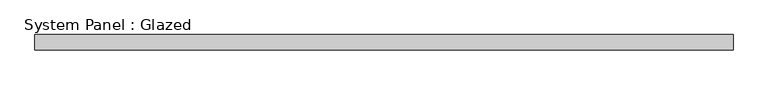
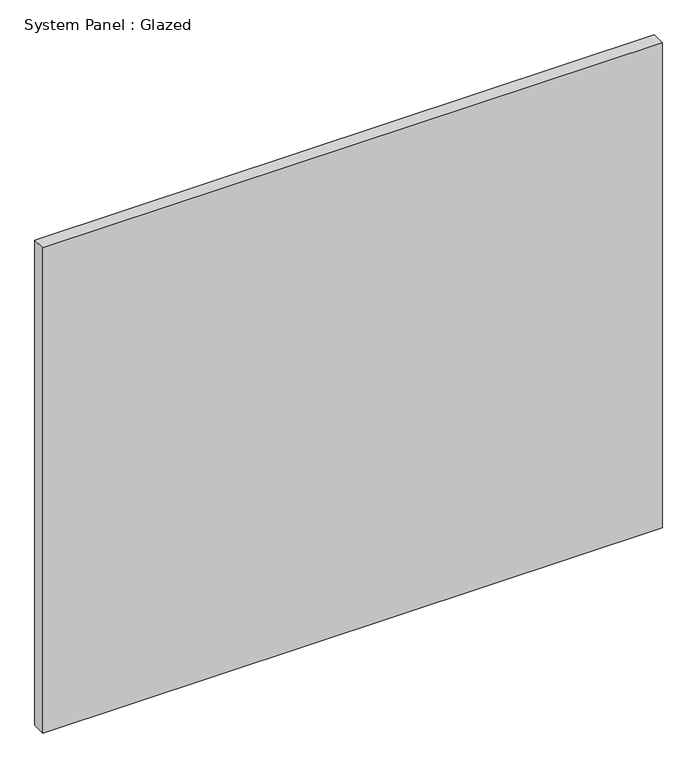
"""IFC4 building model written with IfcOpenShell, lengths in millimetres: plate geometry, System Panel : Glazed."""

from ifc_helpers import new_model, si_unit, origin, origin_with_axes, place, context, project, spatial, polyline, outline, extrude, source, transform, mapped, element, save


def system_panel_glazed_f13871fb(model_context):
    return source(origin(), model_context, "Body", "SweptSolid", [
        extrude(outline(polyline([(577.85, 19.05), (-577.85, 19.05), (-577.85, 44.45), (577.85, 44.45), (577.85, 19.05)])), origin_with_axes(), (0.0, 0.0, 1.0), 956.453622),
    ])


if __name__ == "__main__":
    model = new_model("IFC4")
    model_context = context("Model", 3, world=origin())
    ifc_project = project(units=[si_unit("LENGTHUNIT", "METRE", prefix="MILLI")], contexts=[model_context])
    site = spatial("IfcSite", under=ifc_project)
    building = spatial("IfcBuilding", under=site)
    placement = place(None, origin())
    system_panel_glazed_shape = system_panel_glazed_f13871fb(model_context)
    element("IfcPlate", 1, ObjectType="System Panel : Glazed", at=placement, inside=building, context=model_context, shape_type="MappedRepresentation", body=[
        mapped(system_panel_glazed_shape, transform((0.0, 0.0, 0.0), x_axis=(1.0, 0.0, 0.0), y_axis=(0.0, 1.0, 0.0), z_axis=(0.0, 0.0, 1.0))),
    ])
    save(model, "model.ifc")

# Revit data of these elements
# Type "System Panel : Glazed"
#   Construction Type Id = "GSP4R"
#   Analytic Construction = "1/8 in Pilkington single glazing"
#   Visual Light Transmittance = 0.9
#   Solar Heat Gain Coefficient = 0.86
#   Heat Transfer Coefficient (U) = 1.18115 BTU/(h·ft²·°F)
#   Define Thermal Properties by = 1
# Element 1 (IfcPlate, "System Panel : Glazed")
#   Materials on its faces: "Glass"
# Materials
#   "Glass": class "Glass", colour RGB 0 128 192, transparency 0.75, Description = "Soda Lime Glass", Cost = 0
